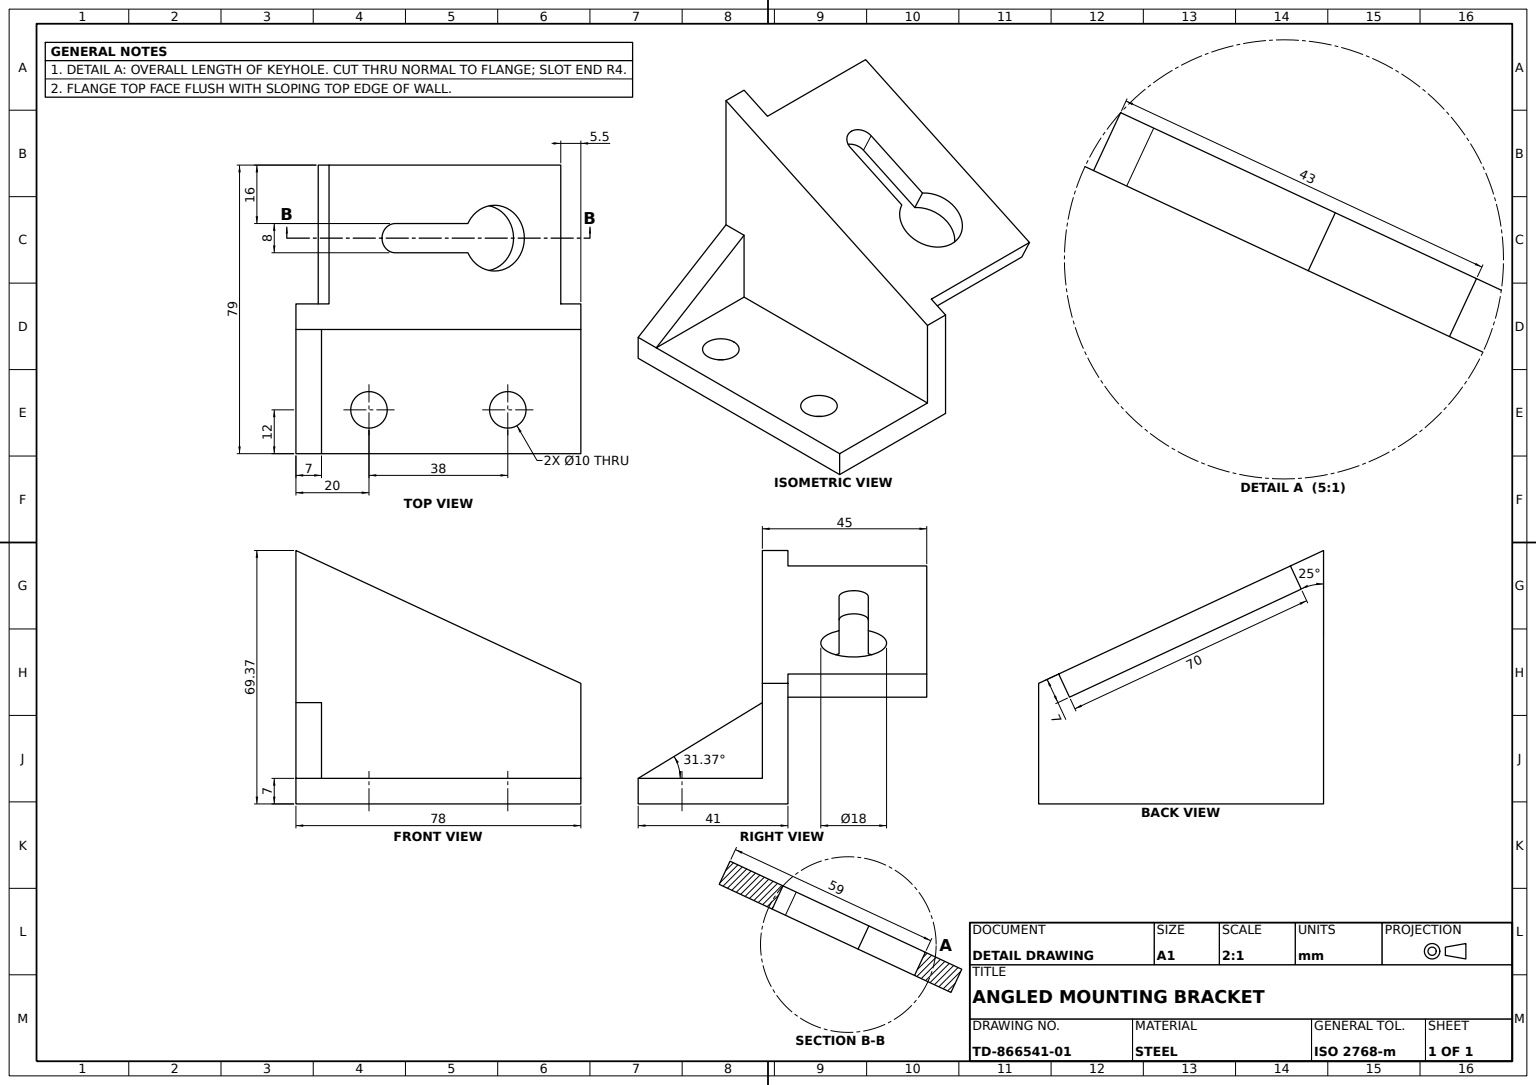
from build123d import *

# Parameters (mm, degrees)
BASE_PLATE_SKETCH_W           = 78
BASE_PLATE_SKETCH_H           = 41
BASE_PLATE_SKETCH_R           = 5
BASE_PLATE_DEPTH              = 7
GUSSET_DEPTH                  = 7
UPRIGHT_WALL_DEPTH            = 7
KEYHOLE_FLANGE_SKETCH_W       = 70
KEYHOLE_FLANGE_SKETCH_H       = 38
KEYHOLE_MOUNTING_FLANGE_DEPTH = 7


with BuildPart() as part:
    # Base Plate Sketch → Base Plate (new body)
    with BuildSketch(Plane(origin=(0, 0, 0), x_dir=(1, 0, 0), z_dir=(0, 1, 0))):
        Rectangle(BASE_PLATE_SKETCH_W, BASE_PLATE_SKETCH_H)
        with Locations(Location((-19, -8.5, 0), (0, 0, 270))):
            Circle(BASE_PLATE_SKETCH_R, mode=Mode.SUBTRACT)
        with Locations(Location((19, -8.5, 0), (0, 0, 270))):
            Circle(BASE_PLATE_SKETCH_R, mode=Mode.SUBTRACT)
    extrude(amount=BASE_PLATE_DEPTH)

    # Gusset Sketch → Gusset (add)
    with BuildSketch(Plane.ZY.offset(39)):
        Polygon((-20.5, 7), (-20.5, 32), (20.5, 7), align=None)
    extrude(amount=-GUSSET_DEPTH)

    # Upright Wall Sketch → Upright Wall (add)
    with BuildSketch(Plane(origin=(0, 0, -20.5), x_dir=(-1, 0, 0), z_dir=(0, 0, -1))):
        Polygon((-39, 7), (-39, 33), (39, 69.371997336), (39, 7), align=None)
    extrude(amount=-UPRIGHT_WALL_DEPTH)

    # Keyhole Flange Sketch → Keyhole Mounting Flange (add)
    with BuildSketch(Plane(origin=(19.605374923, 42.043862201, 0), x_dir=(0.9063077870366493, -0.4226182617407009, 0), z_dir=(0.4226182617407009, 0.9063077870366493, 0))):
        with Locations((-19.663876622, 39.5)):
            Rectangle(KEYHOLE_FLANGE_SKETCH_W, KEYHOLE_FLANGE_SKETCH_H)
        with BuildLine():
            Line((-34.663876622, 42.5), (-12.72613437, 42.5))
            ThreePointArc((-12.72613437, 42.5), (4.336123378, 38.5), (-12.72613437, 34.5))
            Line((-12.72613437, 34.5), (-34.663876622, 34.5))
            ThreePointArc((-34.663876622, 34.5), (-38.663876622, 38.5), (-34.663876622, 42.5))
        make_face(mode=Mode.SUBTRACT)
    extrude(amount=-KEYHOLE_MOUNTING_FLANGE_DEPTH)


solid = part.part
